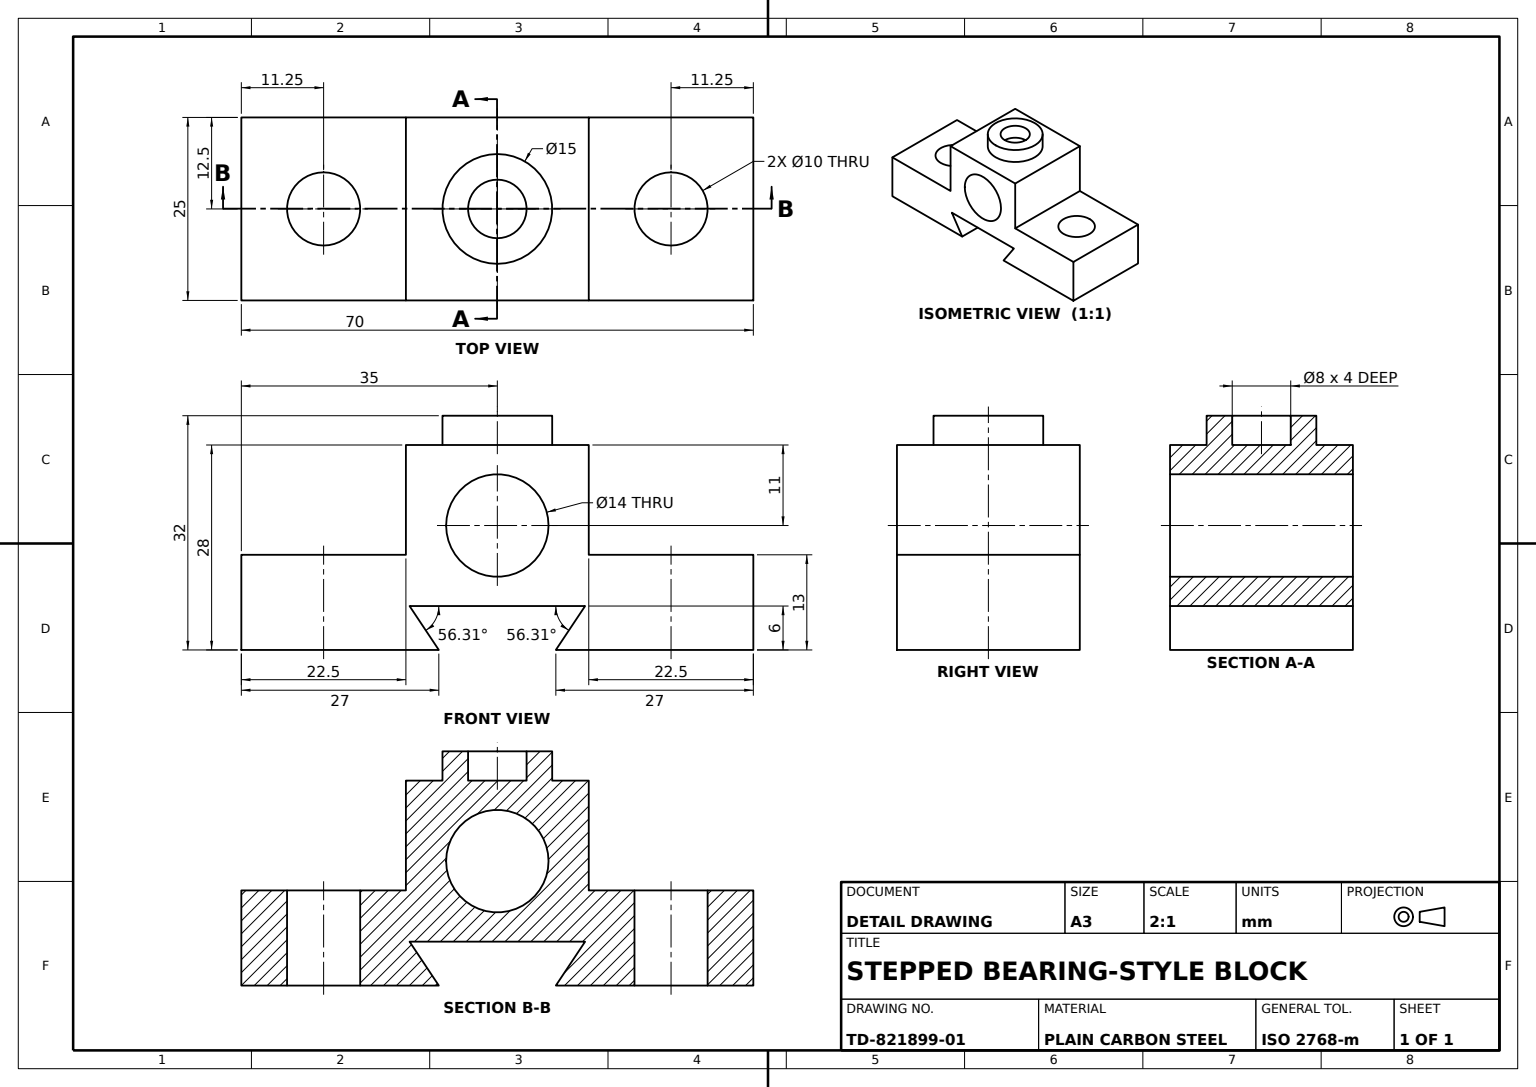
from build123d import *

# Parameters (mm, degrees)
STEPPED_BLOCK_DEPTH          = 25
CROSS_HOLE_SKETCH_R          = 7
CROSS_HOLE_11_DEPTH          = 25
STEP_HOLES_SKETCH_R          = 5
STEP_HOLES_2X_DEPTH_13_DEPTH = 13
TOP_BOSS_SKETCH_R            = 7.5
TOP_BOSS_DEPTH               = 4
TOP_BOSS_BORE_SKETCH_R       = 4
TOP_BOSS_BORE_DEPTH          = 4


with BuildPart() as part:
    # Stepped Block Profile → Stepped Block (new body)
    with BuildSketch(Plane.XY):
        Polygon((0, 0), (0, 13), (22.5, 13), (22.5, 28), (35, 28), (47.5, 28), (47.5, 13), (70, 13), (70, 0), (43, 0), (47, 6), (35, 6), (23, 6), (27, 0), align=None)
    extrude(amount=STEPPED_BLOCK_DEPTH)

    # Cross Hole Sketch → Cross Hole Ø11 (cut)
    with BuildSketch(Plane.XY.offset(25)):
        with Locations((35, 17)):
            Circle(CROSS_HOLE_SKETCH_R)
    extrude(amount=-CROSS_HOLE_11_DEPTH, mode=Mode.SUBTRACT)

    # Step Holes Sketch → Step Holes 2x Depth 13 (cut)
    with BuildSketch(Plane(origin=(0, 13, 0), x_dir=(1, 0, 0), z_dir=(0, 1, 0))):
        with Locations(Location((58.75, -12.5, 0), (0, 0, 270))):
            Circle(STEP_HOLES_SKETCH_R)
        with Locations(Location((11.25, -12.5, 0), (0, 0, 270))):
            Circle(STEP_HOLES_SKETCH_R)
    extrude(amount=-STEP_HOLES_2X_DEPTH_13_DEPTH, mode=Mode.SUBTRACT)

    # Top Boss Sketch → Top Boss (add)
    with BuildSketch(Plane(origin=(0, 28, 0), x_dir=(1, 0, 0), z_dir=(0, 1, 0))):
        with Locations(Location((35, -12.5, 0), (0, 0, 270))):
            Circle(TOP_BOSS_SKETCH_R)
    extrude(amount=TOP_BOSS_DEPTH)

    # Top Boss Bore Sketch → Top Boss Bore (cut)
    with BuildSketch(Plane(origin=(0, 32, 0), x_dir=(1, 0, 0), z_dir=(0, 1, 0))):
        with Locations(Location((35, -12.5, 0), (0, 0, 270))):
            Circle(TOP_BOSS_BORE_SKETCH_R)
    extrude(amount=-TOP_BOSS_BORE_DEPTH, mode=Mode.SUBTRACT)


solid = part.part
